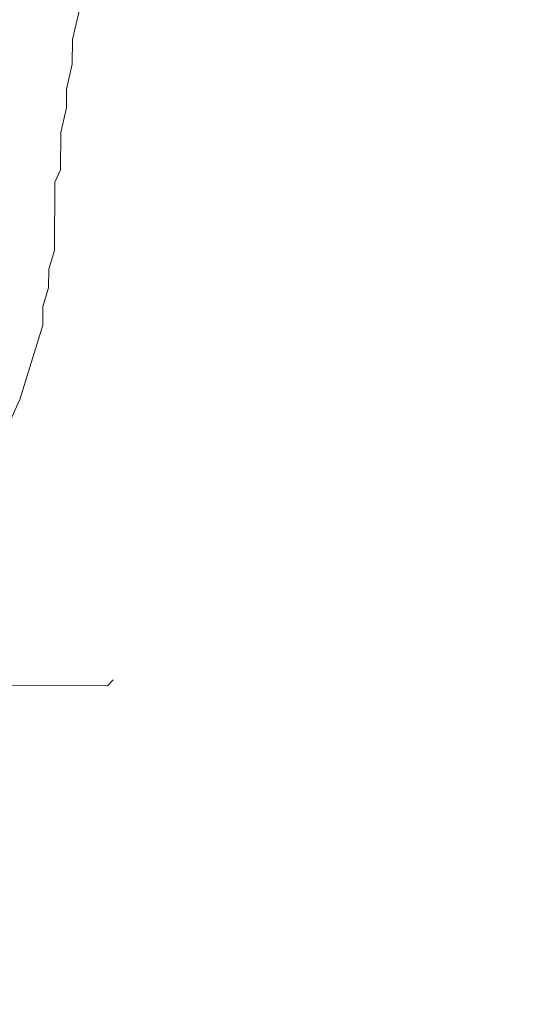
# Model space of a CAD drawing. Units: inches. Extents: x -466983 to 1020, y 324 to 318697.
# Tile 80 of 97: x 660.579 to 662.966, y 939.297 to 944.006. Entities that reach past the tile are written whole.
import ezdxf

# ---------------------------------------------------------------- set-up
doc = ezdxf.new("R2010")
doc.units = ezdxf.units.IN
doc.header["$MEASUREMENT"] = 0
doc.layers.add('A-FLOR-PATT', color=252, linetype='Continuous', lineweight=13)
doc.layers.add('A-FURN', color=8, linetype='Continuous', lineweight=18)

# ---------------------------------------------------------------- blocks, each defined once
blk = doc.blocks.new('L Shaped Sofa')
at = {"ltscale": 2}
for p, q in [((2387.3023, 747.1038), (2387.3515, 747.1578)), ((2387.3515, 747.1578), (2388.5226, 747.1523)), ((2388.1169, 744.6602), (2388.2158, 744.8766)), ((2387.9178, 744.0105), (2388.1169, 744.6602)), ((2387.9168, 743.8479), (2387.9178, 744.0105)), ((2387.867, 743.6855), (2387.9168, 743.8479)), ((2387.866, 743.5228), (2387.867, 743.6855)), ((2387.8162, 743.3604), (2387.866, 743.5228)), ((2387.8125, 742.764), (2387.8162, 743.3604)), ((2387.7631, 742.6558), (2387.8125, 742.764)), ((2387.7611, 742.3305), (2387.7631, 742.6558)), ((2387.711, 742.1139), (2387.7611, 742.3305)), ((2387.71, 741.9512), (2387.711, 742.1139)), ((2387.6598, 741.7346), (2387.71, 741.9512)), ((2387.6585, 741.5177), (2387.6598, 741.7346)), ((2387.5583, 741.0845), (2387.6585, 741.5177))]:
    blk.add_line(p, q, dxfattribs=at)

msp = doc.modelspace()

# ---------------------------------------------------------------- hatches: boundary and pattern name
at = {"layer": 'A-FLOR-PATT', "transparency": 33554572}
h = msp.add_hatch(dxfattribs=at)
h.set_pattern_fill('ANSI37', color=256, scale=30)
h.set_pattern_definition([(45, (-1212.4137, -290.035), (-2.6516504, 2.6516504), []), (135, (-1212.4137, -290.035), (-2.6516504, -2.6516504), [])])
h.paths.add_polyline_path([(901.8057, 1075.9377), (900.6144, 1075.9377), (900.6144, 1065.3856), (899.391, 1065.3856), (898.0911, 1065.3856), (892.8356, 1058.7098, -0.258377), (892.1875, 1058.3509), (879.9848, 1058.3509, -0.20177), (879.4382, 1058.5808), (874.0812, 1065.3856), (872.7813, 1065.3856), (871.5579, 1065.3856), (871.5579, 1075.9377), (813.8057, 1075.9377), (813.8057, 1044.7922), (832.3947, 1044.7922, -0.394795), (848.6602, 1028.5356), (848.6602, 1009.9377), (901.8057, 1009.9377), (901.8057, 1015.9377), (901.3057, 1015.9377), (871.3057, 1015.9377), (871.3057, 1017.2502), (871.3344, 1017.2502, -0.401453), (901.3057, 1045.9377), (901.8057, 1045.9377)])
edge = h.paths.add_edge_path(flags=16)
edge.add_line((847.7731, 1068.9486), (847.7731, 1073.7088))
edge.add_arc((849.2269, 1073.7088), 1.4538, 90, 180, ccw=False)
edge.add_line((849.2269, 1075.1627), (864.4921, 1075.1627))
edge.add_arc((864.4921, 1073.7088), 1.4538, 0, 90, ccw=False)
edge.add_line((865.9459, 1073.7088), (865.9459, 1069.0035))
edge.add_arc((832.6447, 1068.9761), 33.3012, -20.61234, 0.04725, ccw=False)
edge.add_ellipse((856.8595, 1058.48), major_axis=(0, 10.2131), ratio=0.6859192, start_angle=100.00884, end_angle=259.99116, ccw=False)
edge.add_arc((881.0742, 1068.9761), 33.3012, 180.04725, 200.61234, ccw=False)
h.paths.add_polyline_path([(853.1456, 1066.4815), (853.1456, 1066.4534), (853.1463, 1066.4534, 0.433107), (852.9166, 1066.6849), (852.9166, 1066.4534), (853.1456, 1066.4534), (853.1456, 1066.4815), (853.088, 1066.6122, 0.697939), (852.6995, 1066.4534), (852.7003, 1066.4534), (852.7003, 1066.4815), (852.9166, 1067.0012), (852.9166, 1066.6849, -0.396254)], flags=0)
h.paths.add_polyline_path([(861.0187, 1066.4815), (861.0187, 1066.4534), (861.0194, 1066.4534, 0.416404), (860.8024, 1066.6849), (860.8024, 1066.4534), (861.0187, 1066.4534), (861.0187, 1066.4815), (860.9672, 1066.6053, 0.713344), (860.5726, 1066.4534), (860.5734, 1066.4534), (860.5734, 1066.4815), (860.8024, 1067.0012), (860.8024, 1066.6849, -0.379973)], flags=0)
edge = h.paths.add_edge_path(flags=0)
edge.add_spline(control_points=[(861.1298, 1065.7855), (861.4661, 1065.2478), (861.6134, 1065.0161), (861.9833, 1064.3736), (862.1924, 1063.9443), (862.5614, 1063.0391), (862.7212, 1062.5633), (862.9865, 1061.5781), (863.092, 1061.0689), (863.2452, 1060.031), (863.293, 1059.5025), (863.3295, 1058.4409), (863.3181, 1057.9078), (863.2366, 1056.8518), (863.1664, 1056.3289), (862.9695, 1055.308), (862.8427, 1054.8099), (862.5365, 1053.8522), (862.3571, 1053.3927), (861.9514, 1052.5249), (861.7251, 1052.1166), (861.233, 1051.3622), (860.9672, 1051.0162), (860.4048, 1050.3949), (860.1082, 1050.1197), (859.4937, 1049.6461), (859.1758, 1049.4476), (858.5276, 1049.1299), (858.1973, 1049.0107), (857.5315, 1048.8518), (857.1959, 1048.8121), (856.5249, 1048.812), (856.1894, 1048.8515), (855.5236, 1049.0101), (855.1933, 1049.1291), (854.545, 1049.4465), (854.2271, 1049.6449), (853.6124, 1050.1183), (853.3158, 1050.3933), (852.7533, 1051.0143), (852.4874, 1051.3602), (851.9952, 1052.1144), (851.7688, 1052.5225), (851.3629, 1053.3902), (851.1834, 1053.8496), (850.877, 1054.8071), (850.7501, 1055.3051), (850.553, 1056.326), (850.4827, 1056.8488), (850.401, 1057.9048), (850.3895, 1058.4379), (850.4257, 1059.4995), (850.4734, 1060.0281), (850.6265, 1061.066), (850.7318, 1061.5753), (850.9969, 1062.5605), (851.1567, 1063.0365), (851.5254, 1063.9418), (851.7345, 1064.3712), (852.1056, 1065.0164), (852.2544, 1065.2503), (852.6082, 1065.7335)], knot_values=[3.915332, 3.915332, 3.915332, 3.915332, 4.013468, 4.013468, 4.175532, 4.175532, 4.337596, 4.337596, 4.49966, 4.49966, 4.661724, 4.661724, 4.823788, 4.823788, 4.985852, 4.985852, 5.147916, 5.147916, 5.30998, 5.30998, 5.472044, 5.472044, 5.634109, 5.634109, 5.796173, 5.796173, 5.958237, 5.958237, 6.120301, 6.120301, 6.282365, 6.282365, 6.444429, 6.444429, 6.606493, 6.606493, 6.768557, 6.768557, 6.930621, 6.930621, 7.092685, 7.092685, 7.254749, 7.254749, 7.416813, 7.416813, 7.578878, 7.578878, 7.740942, 7.740942, 7.903006, 7.903006, 8.06507, 8.06507, 8.227134, 8.227134, 8.389198, 8.389198, 8.551262, 8.551262, 8.65037, 8.65037, 8.65037, 8.65037], degree=3, periodic=0)
edge.add_line((852.6421, 1065.7855), (861.1298, 1065.7855))
edge = h.paths.add_edge_path(flags=0)
edge.add_ellipse((856.8496, 1057.7432), major_axis=(0, 7.7921), ratio=0.687861, start_angle=0, end_angle=360)
h.paths.add_polyline_path([(848.8634, 1069.3891), (848.8634, 1073.9605, -0.414214), (849.9538, 1075.0508), (863.7652, 1075.0508, -0.414214), (864.8555, 1073.9605), (864.8555, 1069.3891, -0.388936), (864.5237, 1069.027, -0.043561), (849.1953, 1069.027, -0.388936)], flags=0)
h.paths.add_polyline_path([(853.1006, 1068.1122, -1), (852.6775, 1068.1122, -1)], flags=0)
edge = h.paths.add_edge_path(flags=0)
edge.add_ellipse((856.8595, 1057.3378), major_axis=(0, 2.207), ratio=0.657164, start_angle=0, end_angle=360)
h.paths.add_polyline_path([(861.0415, 1068.1122, -1), (860.6184, 1068.1122, -1)], flags=0)
edge = h.paths.add_edge_path()
edge.add_line((573.9537, 1057.3412), (573.9537, 1075.9377))
edge.add_line((573.9537, 1075.9377), (558.7308, 1075.9377))
edge.add_line((558.7308, 1075.9377), (558.7308, 1065.3856))
edge.add_line((558.7308, 1065.3856), (557.5074, 1065.3856))
edge.add_line((557.5074, 1065.3856), (556.2075, 1065.3856))
edge.add_line((556.2075, 1065.3856), (550.952, 1058.7098))
edge.add_arc((550.3039, 1059.1155), 0.7646, 270, 327.9483, ccw=False)
edge.add_line((550.3039, 1058.3509), (538.1012, 1058.3509))
edge.add_arc((538.1012, 1059.1155), 0.7646, 224.3704, 270, ccw=False)
edge.add_line((537.5546, 1058.5808), (532.1976, 1065.3856))
edge.add_line((532.1976, 1065.3856), (530.8977, 1065.3856))
edge.add_line((530.8977, 1065.3856), (529.6743, 1065.3856))
edge.add_line((529.6743, 1065.3856), (529.6743, 1075.9377))
edge.add_line((529.6743, 1075.9377), (520.8057, 1075.9377))
edge.add_line((520.8057, 1075.9377), (520.8057, 1045.9377))
edge.add_line((520.8057, 1045.9377), (521.3057, 1045.9377))
edge.add_arc((521.3057, 1015.9377), 30, 2.50749, 90, ccw=False)
edge.add_line((551.277, 1017.2502), (551.3057, 1017.2502))
edge.add_line((551.3057, 1017.2502), (551.3057, 1015.9377))
edge.add_line((551.3057, 1015.9377), (520.8057, 1015.9377))
edge.add_line((520.8057, 1015.9377), (520.8057, 1009.9377))
edge.add_line((520.8057, 1009.9377), (559.1913, 1010.4022))
edge.add_arc((559.1913, 1011.856), 1.4538, 180, 270, ccw=False)
edge.add_line((557.7375, 1011.856), (557.7375, 1016.5613))
edge.add_arc((591.0386, 1016.5888), 33.3012, 159.38766, 180.04725, ccw=False)
edge.add_ellipse((566.8239, 1027.0848), major_axis=(0, 10.2131), ratio=0.6859192, start_angle=280.00884, end_angle=439.99116, ccw=False)
edge.add_arc((542.6091, 1016.5888), 33.3012, 0.04725, 20.61234, ccw=False)
edge.add_line((575.9103, 1016.6162), (575.9103, 1011.856))
edge.add_arc((574.4565, 1011.856), 1.4538, -90, 0, ccw=False)
edge.add_line((574.4565, 1010.4022), (608.8057, 1009.9377))
edge.add_line((608.8057, 1009.9377), (608.8057, 1041.0857))
edge.add_line((608.8057, 1041.0857), (590.2179, 1041.0857))
edge.add_arc((590.775, 1057.9074), 16.8309, 181.92775, 268.10321, ccw=False)
edge = h.paths.add_edge_path()
edge.add_ellipse((494.2443, 583.6204), major_axis=(0, 10.2131), ratio=0.6859192, start_angle=280.00884, end_angle=439.99116, ccw=False)
edge.add_arc((470.0296, 573.1243), 33.3012, 0.04725, 20.61234, ccw=False)
edge.add_line((503.3307, 573.1518), (503.3307, 568.3916))
edge.add_arc((501.8769, 568.3916), 1.4538, -90, 0, ccw=False)
edge.add_line((501.8769, 566.9377), (539.8057, 566.9377))
edge.add_line((539.8057, 566.9377), (539.8057, 572.9377))
edge.add_line((539.8057, 572.9377), (539.3057, 572.9377))
edge.add_line((539.3057, 572.9377), (509.3057, 572.9377))
edge.add_line((509.3057, 572.9377), (509.3057, 574.2502))
edge.add_line((509.3057, 574.2502), (509.3344, 574.2502))
edge.add_arc((539.3057, 572.9377), 30, 90, 177.49251, ccw=False)
edge.add_line((539.3057, 602.9377), (539.8057, 602.9377))
edge.add_line((539.8057, 602.9377), (539.8057, 626.9377))
edge.add_line((539.8057, 626.9377), (531.7718, 626.9377))
edge.add_line((531.7718, 626.9377), (531.7718, 616.3856))
edge.add_line((531.7718, 616.3856), (530.5484, 616.3856))
edge.add_line((530.5484, 616.3856), (529.2485, 616.3856))
edge.add_line((529.2485, 616.3856), (523.7105, 609.3509))
edge.add_line((523.7105, 609.3509), (510.7766, 609.3509))
edge.add_line((510.7766, 609.3509), (505.2386, 616.3856))
edge.add_line((505.2386, 616.3856), (503.9387, 616.3856))
edge.add_line((503.9387, 616.3856), (502.7153, 616.3856))
edge.add_line((502.7153, 616.3856), (502.7153, 626.9377))
edge.add_line((502.7153, 626.9377), (481.6983, 626.9377))
edge.add_line((481.6983, 626.9377), (481.6983, 610.995))
edge.add_arc((467.2703, 611.4728), 14.4359, 271.92775, 358.10321, ccw=False)
edge.add_line((467.7559, 597.0451), (451.8057, 597.0451))
edge.add_line((451.8057, 597.0451), (451.8057, 584.4035))
edge.add_line((451.8057, 584.4035), (451.8057, 566.9377))
edge.add_line((451.8057, 566.9377), (486.6117, 566.9377))
edge.add_arc((486.6117, 568.3916), 1.4538, 180, 270, ccw=False)
edge.add_line((485.1579, 568.3916), (485.1579, 573.0969))
edge.add_arc((518.4591, 573.1243), 33.3012, 159.38766, 180.04725, ccw=False)
h.paths.add_polyline_path([(836.2609, 1020.7328), (879.8898, 1020.7328), (879.8898, 1039.3902), (836.2609, 1039.3902)], flags=25)
h.paths.add_polyline_path([(549.9851, 1036.7492), (593.614, 1036.7492), (593.614, 1055.4065), (549.9851, 1055.4065)], flags=24)
h.paths.add_polyline_path([(475.123, 595.5959), (518.752, 595.5959), (518.752, 614.2532), (475.123, 614.2532)], flags=24)
h = msp.add_hatch(dxfattribs=at)
h.set_pattern_fill('ANSI37', color=256, scale=20)
h.set_pattern_definition([(45, (-1212.4137, -290.035), (-1.767767, 1.767767), []), (135, (-1212.4137, -290.035), (-1.767767, -1.767767), [])])
h.paths.add_polyline_path([(809.8057, 870.9377), (809.8057, 888.1519), (806.9985, 888.1519), (802.6624, 888.1519), (789.3832, 888.1519), (786.2846, 888.1519, -0.414214), (785.4991, 888.9374), (785.4991, 900.1959), (785.4991, 908.4696, -0.414214), (786.8082, 909.7787, -0.414214), (785.4991, 911.0878), (785.4991, 929.1015, -0.414214), (786.8082, 930.4106, -0.414214), (785.4991, 931.7197), (785.4991, 931.9039, -0.414214), (784.19, 930.5948), (766.7223, 930.5948, -0.412359), (765.4132, 931.8956, -0.413741), (764.1145, 930.5782), (744.5781, 930.422, -0.416556), (743.7864, 931.2075), (743.7864, 933.5153), (742.2154, 933.5153), (742.2154, 952.024, -0.001344), (743.7864, 952.1998), (743.7864, 953.9377), (678.5915, 953.9377), (678.5915, 951.1305), (678.5915, 946.7945), (678.5915, 933.5153), (678.5915, 930.4166, -0.414214), (677.806, 929.6312), (666.5475, 929.6312), (658.2738, 929.6312, -0.414214), (656.9647, 930.9403, -0.414214), (655.6556, 929.6312), (637.6419, 929.6312, -0.414214), (636.3328, 930.9403, -0.414214), (635.0237, 929.6312), (634.8395, 929.6312, -0.414214), (636.1486, 928.322), (636.1486, 910.8544, -0.412359), (634.8478, 909.5452, -0.413741), (636.1653, 908.2466), (636.3214, 888.7102, -0.416556), (635.5359, 887.9184), (633.2281, 887.9184), (633.2281, 886.3475), (614.7194, 886.3475, -0.001344), (614.5436, 887.9184), (612.8057, 887.9184), (612.8057, 834.9377), (612.8057, 752.9377), (612.8057, 748.9377), (612.8057, 697.9377), (654.8057, 697.9377), (654.8057, 701.9377), (715.8057, 701.9377), (715.8057, 737.4353), (774.2918, 737.4353), (774.2918, 795.9377), (809.8057, 795.9377)])
h.paths.add_polyline_path([(679.2761, 849.5757, 0.102523), (682.1475, 849.2608, -0.080461), (694.5428, 849.7725, -0.283899), (694.4822, 849.0082, 0.136605), (694.4068, 848.8103, -0.030441), (694.5428, 846.8929), (694.5428, 842.6198), (694.5428, 838.3466, -0.028219), (694.4246, 836.5684), (694.425, 836.5684, 0.196187), (694.4456, 836.2708, -0.302897), (694.5428, 835.467, -0.080461), (682.1475, 835.9787, 0.102523), (679.2761, 835.6638, -0.58611), (678.6457, 836.0169), (678.6457, 849.2227, -0.58611)], flags=16)
h.paths.add_polyline_path([(679.5173, 848.6515, 0.699597), (679.476, 848.6342, 1.20716), (679.1935, 848.7422, 0.010621)], flags=0)
h.paths.add_polyline_path([(679.4923, 836.5608, -0.013798), (679.9178, 836.6594, -0.071703), (682.8533, 837.1434, -0.165743), (682.1665, 839.1006), (682.1665, 842.6094), (682.1665, 846.0603, -0.240616), (683.4733, 848.6767, -0.068263), (693.9295, 849.0082), (693.7875, 848.7083), (693.7875, 849.0228, 0.067332), (683.4733, 848.6767, 0.240616), (682.1665, 846.0603), (682.1665, 842.6094), (682.1665, 839.1006, 0.23459), (683.461, 836.5513, 0.068093), (693.7875, 836.1955), (693.7875, 836.5104), (693.9296, 836.2102, -0.077215), (682.2421, 836.7815, 0.086627), (679.5283, 836.5701, -0.628402), (679.5029, 836.5735), (679.5029, 836.6071, 0.910458)], flags=0)
h.paths.add_polyline_path([(679.476, 848.6364), (679.2069, 848.647), (679.2069, 836.5718, 0.913566), (679.3645, 836.5861), (679.476, 836.5824)], flags=0)
h.paths.add_polyline_path([(679.2761, 829.8604, 0.102523), (682.1475, 829.5455, -0.080461), (694.5428, 830.0572, -0.283899), (694.4822, 829.2929, 0.136605), (694.4068, 829.095, -0.030441), (694.5428, 827.1776), (694.5428, 822.9045), (694.5428, 818.6314, -0.028219), (694.4246, 816.8531), (694.425, 816.8532, 0.196187), (694.4456, 816.5555, -0.302897), (694.5428, 815.7517, -0.080461), (682.1475, 816.2635, 0.102523), (679.2761, 815.9485, -0.58611), (678.6457, 816.3016), (678.6457, 829.5074, -0.58611)], flags=16)
h.paths.add_polyline_path([(679.5173, 828.9362, 0.699597), (679.476, 828.9189, 1.20716), (679.1935, 829.0269, 0.010621)], flags=0)
h.paths.add_polyline_path([(679.4923, 816.8456, -0.013798), (679.9178, 816.9441, -0.071703), (682.8533, 817.4281, -0.165743), (682.1665, 819.3853), (682.1665, 822.8941), (682.1665, 826.345, -0.240616), (683.4733, 828.9614, -0.068263), (693.9295, 829.2929), (693.7875, 828.9931), (693.7875, 829.3076, 0.067332), (683.4733, 828.9614, 0.240616), (682.1665, 826.345), (682.1665, 822.8941), (682.1665, 819.3853, 0.23459), (683.461, 816.836, 0.068093), (693.7875, 816.4802), (693.7875, 816.7952), (693.9296, 816.4949, -0.077215), (682.2421, 817.0662, 0.086627), (679.5283, 816.8549, -0.628402), (679.5029, 816.8582), (679.5029, 816.8918, 0.910458)], flags=0)
h.paths.add_polyline_path([(679.476, 828.9211), (679.2069, 828.9317), (679.2069, 816.8565, 0.913566), (679.3645, 816.8708), (679.476, 816.8671)], flags=0)
h.paths.add_polyline_path([(679.2761, 810.1451, 0.102523), (682.1475, 809.8302, -0.080461), (694.5428, 810.342, -0.3023), (694.4466, 809.5394, 0.10023), (694.4058, 809.3878, -0.03057), (694.5428, 807.4623), (694.5428, 803.1892), (694.5428, 798.9161, -0.03057), (694.4058, 796.9906, 0.10023), (694.4466, 796.839, -0.3023), (694.5428, 796.0365, -0.080461), (682.1475, 796.5482, 0.102523), (679.2761, 796.2333, -0.58611), (678.6457, 796.5863), (678.6457, 809.7921, -0.58611)], flags=16)
h.paths.add_polyline_path([(679.5173, 809.2417, 0.699597), (679.476, 809.2244, 1.20716), (679.1935, 809.3324, 0.010621)], flags=0)
h.paths.add_polyline_path([(679.4923, 797.151, -0.013798), (679.9178, 797.2496, -0.071703), (682.8533, 797.7336, -0.165743), (682.1665, 799.6908), (682.1665, 803.1996), (682.1665, 806.6505, -0.239349), (683.461, 809.2577, -0.072465), (694.4468, 809.5405, 0.197932), (694.425, 809.2405), (693.7875, 809.2985), (693.7875, 809.6135, 0.068093), (683.461, 809.2577, 0.239349), (682.1665, 806.6505), (682.1665, 803.1996), (682.1665, 799.6908, 0.235854), (683.4733, 797.1323, 0.067332), (693.7875, 796.7861), (693.7875, 797.1006), (694.425, 797.1586, 0.197932), (694.4468, 796.8586, -0.080419), (682.1557, 797.3795, 0.083867), (679.5283, 797.1603, -0.628402), (679.5029, 797.1637), (679.5029, 797.1973, 0.910458)], flags=0)
h.paths.add_polyline_path([(679.2069, 809.2372), (679.2069, 797.162, 0.913566), (679.3645, 797.1763), (679.476, 797.1726), (679.476, 809.2266)], flags=0)
h.paths.add_polyline_path([(695.3643, 853.2989), (728.2231, 853.2989), (728.2231, 771.1519), (695.3643, 771.1519)], flags=16)
h.paths.add_polyline_path([(696.0215, 852.6417), (727.5659, 852.6417), (727.5659, 771.809), (696.0215, 771.809)], flags=0)
h.paths.add_polyline_path([(679.2761, 788.7869, 0.102523), (682.1475, 788.472, -0.080461), (694.5428, 788.9837, -0.3023), (694.4466, 788.1812, 0.10023), (694.4058, 788.0296, -0.03057), (694.5428, 786.1041), (694.5428, 781.831), (694.5428, 777.5578, -0.03057), (694.4058, 775.6323, 0.10023), (694.4466, 775.4808, -0.3023), (694.5428, 774.6782, -0.080461), (682.1475, 775.19, 0.102523), (679.2761, 774.875, -0.58611), (678.6457, 775.2281), (678.6457, 788.4339, -0.58611)], flags=16)
h.paths.add_polyline_path([(679.5173, 787.8834, 0.699597), (679.476, 787.8662, 1.20716), (679.1935, 787.9742, 0.010621)], flags=0)
h.paths.add_polyline_path([(679.4923, 775.7928, -0.013798), (679.9178, 775.8914, -0.071703), (682.8533, 776.3753, -0.165743), (682.1665, 778.3325), (682.1665, 781.8414), (682.1665, 785.2922, -0.239349), (683.461, 787.8995, -0.072465), (694.4468, 788.1823, 0.197932), (694.425, 787.8823), (693.7875, 787.9403), (693.7875, 788.2553, 0.068093), (683.461, 787.8995, 0.239349), (682.1665, 785.2922), (682.1665, 781.8414), (682.1665, 778.3325, 0.235854), (683.4733, 775.7741, 0.067332), (693.7875, 775.4279), (693.7875, 775.7424), (694.425, 775.8004, 0.197932), (694.4468, 775.5004, -0.080419), (682.1557, 776.0212, 0.083867), (679.5283, 775.8021, -0.628402), (679.5029, 775.8054), (679.5029, 775.8391, 0.910458)], flags=0)
h.paths.add_polyline_path([(679.2069, 787.8789), (679.2069, 775.8038, 0.913566), (679.3645, 775.818), (679.476, 775.8144), (679.476, 787.8684)], flags=0)
h.paths.add_polyline_path([(704.641, 854.1204, -0.080461), (705.1527, 866.5157, 0.102523), (704.8378, 869.3871, -0.58611), (705.1908, 870.0174), (718.3966, 870.0174, -0.58611), (718.7496, 869.3871, 0.102523), (718.4347, 866.5157, -0.080461), (718.9465, 854.1204, -0.3023), (718.1439, 854.2166, 0.10023), (717.9924, 854.2574, -0.03057), (716.0668, 854.1204), (711.7937, 854.1204), (707.5206, 854.1204, -0.03057), (705.5951, 854.2574, 0.10023), (705.4435, 854.2166, -0.3023)], flags=16)
h.paths.add_polyline_path([(717.8462, 869.1459, 0.699597), (717.8289, 869.1872, 1.20716), (717.9369, 869.4697, 0.010621)], flags=0)
h.paths.add_polyline_path([(705.4631, 854.2164, -0.080419), (705.984, 866.5074, 0.083867), (705.7648, 869.1349, -0.628402), (705.7682, 869.1603), (705.8018, 869.1603, 0.910458), (705.7555, 869.1709, -0.013798), (705.8541, 868.7454, -0.071703), (706.3381, 865.8099, -0.165743), (708.2953, 866.4967), (711.8041, 866.4967), (715.255, 866.4967, -0.239349), (717.8622, 865.2022, -0.072465), (718.145, 854.2164, 0.197932), (717.845, 854.2382), (717.903, 854.8757), (718.218, 854.8757, 0.068093), (717.8622, 865.2022, 0.239349), (715.255, 866.4967), (711.8041, 866.4967), (708.2953, 866.4967, 0.235854), (705.7368, 865.1898, 0.067332), (705.3906, 854.8757), (705.7051, 854.8757), (705.7631, 854.2382, 0.197932)], flags=16)
h.paths.add_polyline_path([(705.7665, 869.4563, 0.913566), (705.7808, 869.2987), (705.7771, 869.1872), (717.8311, 869.1872), (717.8417, 869.4563)], flags=0)
h.paths.add_polyline_path([(729.0446, 842.6198), (729.0446, 846.8929, -0.03057), (729.1817, 848.8184, 0.10023), (729.1408, 848.9699, -0.3023), (729.0446, 849.7725, -0.080461), (741.4399, 849.2608, 0.102523), (744.3113, 849.5757, -0.58611), (744.9417, 849.2227), (744.9417, 836.0169, -0.58611), (744.3113, 835.6638, 0.102523), (741.4399, 835.9787, -0.080461), (729.0446, 835.467, -0.3023), (729.1408, 836.2696, 0.10023), (729.1817, 836.4211, -0.03057), (729.0446, 838.3466)], flags=16)
h.paths.add_polyline_path([(744.1115, 836.5846, 1.20716), (744.3939, 836.4766, 0.010621), (744.0701, 836.5673, 0.699597)], flags=0)
h.paths.add_polyline_path([(729.1407, 836.2684, 0.197932), (729.1624, 836.5684), (729.7999, 836.5104), (729.7999, 836.1955, 0.068093), (740.1264, 836.5513, 0.239349), (741.4209, 839.1585), (741.4209, 842.6094), (741.4209, 846.1182, 0.235854), (740.1141, 848.6767, 0.067332), (729.7999, 849.0228), (729.7999, 848.7083), (729.1624, 848.6503, 0.197932), (729.1407, 848.9504, -0.080419), (741.4317, 848.4295, 0.083867), (744.0591, 848.6486, -0.628402), (744.0845, 848.6453), (744.0845, 848.6117, 0.910458), (744.0951, 848.6579, -0.013798), (743.6696, 848.5594, -0.071703), (740.7341, 848.0754, -0.165743), (741.4209, 846.1182), (741.4209, 842.6094), (741.4209, 839.1585, -0.239349), (740.1264, 836.5513, -0.072465)], flags=0)
h.paths.add_polyline_path([(729.0446, 830.0572, -0.080461), (741.4399, 829.5455, 0.102523), (744.3113, 829.8604, -0.58611), (744.9417, 829.5074), (744.9417, 816.3016, -0.58611), (744.3113, 815.9485, 0.102523), (741.4399, 816.2635, -0.080461), (729.0446, 815.7517, -0.3023), (729.1408, 816.5543, 0.10023), (729.1817, 816.7058, -0.03057), (729.0446, 818.6314), (729.0446, 822.9045), (729.0446, 827.1776, -0.03057), (729.1817, 829.1031, 0.10023), (729.1408, 829.2547, -0.3023)], flags=16)
h.paths.add_polyline_path([(744.1115, 816.8693, 1.20716), (744.3939, 816.7613, 0.010621), (744.0701, 816.852, 0.699597)], flags=0)
h.paths.add_polyline_path([(729.1407, 829.2351, -0.080419), (741.4317, 828.7142, 0.083867), (744.0591, 828.9334, -0.628402), (744.0845, 828.93), (744.0845, 828.8964, 0.910458), (744.0951, 828.9427, -0.013798), (743.6696, 828.8441, -0.071703), (740.7341, 828.3601, -0.165743), (741.4209, 826.4029), (741.4209, 822.8941), (741.4209, 819.4432, -0.239349), (740.1264, 816.836, -0.072465), (729.1407, 816.5531, 0.197932), (729.1624, 816.8532), (729.7999, 816.7952), (729.7999, 816.4802, 0.068093), (740.1264, 816.836, 0.239349), (741.4209, 819.4432), (741.4209, 822.8941), (741.4209, 826.4029, 0.235854), (740.1141, 828.9614, 0.067332), (729.7999, 829.3076), (729.7999, 828.9931), (729.1624, 828.9351, 0.197932)], flags=16)
h.paths.add_polyline_path([(729.0446, 810.342, -0.080461), (741.4399, 809.8302, 0.102523), (744.3113, 810.1451, -0.58611), (744.9417, 809.7921), (744.9417, 796.5863, -0.58611), (744.3113, 796.2333, 0.102523), (741.4399, 796.5482, -0.080461), (729.0446, 796.0365, -0.283899), (729.1052, 796.8007, 0.136605), (729.1806, 796.9987, -0.030441), (729.0446, 798.9161), (729.0446, 803.1892), (729.0446, 807.4623, -0.028219), (729.1628, 809.2406), (729.1624, 809.2405, 0.196187), (729.1418, 809.5382, -0.302897)], flags=16)
h.paths.add_polyline_path([(744.1115, 797.1748, 1.20716), (744.3939, 797.0668, 0.010621), (744.0701, 797.1575, 0.699597)], flags=0)
h.paths.add_polyline_path([(741.3453, 809.0275, 0.086627), (744.0591, 809.2388, -0.628402), (744.0845, 809.2355), (744.0845, 809.2019, 0.910458), (744.0951, 809.2481, -0.013798), (743.6696, 809.1496, -0.071703), (740.7341, 808.6656, -0.165743), (741.4209, 806.7084), (741.4209, 803.1996), (741.4209, 799.7487, -0.240616), (740.1141, 797.1323, -0.068263), (729.658, 796.8008), (729.7999, 797.1006), (729.7999, 796.7861, 0.067332), (740.1141, 797.1323, 0.240616), (741.4209, 799.7487), (741.4209, 803.1996), (741.4209, 806.7084, 0.23459), (740.1264, 809.2577, 0.068093), (729.7999, 809.6135), (729.7999, 809.2985), (729.6578, 809.5988, -0.077215)], flags=0)
h.paths.add_polyline_path([(704.641, 770.3304, -0.283899), (705.4053, 770.2697, 0.136605), (705.6032, 770.1944, -0.030441), (707.5206, 770.3304), (711.7937, 770.3304), (716.0668, 770.3304, -0.028219), (717.8451, 770.2122), (717.845, 770.2126, 0.196187), (718.1427, 770.2331, -0.302897), (718.9465, 770.3304, -0.080461), (718.4347, 757.9351, 0.102523), (718.7496, 755.0637, -0.58611), (718.3966, 754.4333), (705.1908, 754.4333, -0.58611), (704.8378, 755.0637, 0.102523), (705.1527, 757.9351, -0.080461)], flags=16)
h.paths.add_polyline_path([(705.762, 755.3048, 0.699597), (705.7793, 755.2635, 1.20716), (705.6713, 754.9811, 0.010621)], flags=0)
h.paths.add_polyline_path([(705.4053, 769.717), (705.7051, 769.5751), (705.3906, 769.5751, 0.067332), (705.7368, 759.2609, 0.240616), (708.3532, 757.954), (711.8041, 757.954), (715.3129, 757.954, 0.23459), (717.8622, 759.2485, 0.068093), (718.218, 769.5751), (717.903, 769.5751), (718.2033, 769.7172, -0.077215), (717.632, 758.0297, 0.086627), (717.8433, 755.3159, -0.628402), (717.84, 755.2904), (717.8064, 755.2904, 0.910458), (717.8526, 755.2799, -0.013798), (717.7541, 755.7053, -0.071703), (717.2701, 758.6409, -0.165743), (715.3129, 757.954), (711.8041, 757.954), (708.3532, 757.954, -0.240616), (705.7368, 759.2609, -0.068263)], flags=0)
h.paths.add_polyline_path([(729.0446, 788.9837, -0.080461), (741.4399, 788.472, 0.102523), (744.3113, 788.7869, -0.58611), (744.9417, 788.4339), (744.9417, 775.2281, -0.58611), (744.3113, 774.875, 0.102523), (741.4399, 775.19, -0.080461), (729.0446, 774.6782, -0.283899), (729.1052, 775.4425, 0.136605), (729.1806, 775.6405, -0.030441), (729.0446, 777.5578), (729.0446, 781.831), (729.0446, 786.1041, -0.028219), (729.1628, 787.8823), (729.1624, 787.8823, 0.196187), (729.1418, 788.1799, -0.302897)], flags=16)
h.paths.add_polyline_path([(744.1115, 775.8165, 1.20716), (744.3939, 775.7086, 0.010621), (744.0701, 775.7993, 0.699597)], flags=0)
h.paths.add_polyline_path([(741.3453, 787.6692, 0.086627), (744.0591, 787.8806, -0.628402), (744.0845, 787.8773), (744.0845, 787.8437, 0.910458), (744.0951, 787.8899, -0.013798), (743.6696, 787.7913, -0.071703), (740.7341, 787.3074, -0.165743), (741.4209, 785.3502), (741.4209, 781.8414), (741.4209, 778.3905, -0.240616), (740.1141, 775.7741, -0.068263), (729.658, 775.4425), (729.7999, 775.7424), (729.7999, 775.4279, 0.067332), (740.1141, 775.7741, 0.240616), (741.4209, 778.3905), (741.4209, 781.8414), (741.4209, 785.3502, 0.23459), (740.1264, 787.8995, 0.068093), (729.7999, 788.2553), (729.7999, 787.9403), (729.6578, 788.2405, -0.077215)], flags=0)
h.paths.add_polyline_path([(744.1115, 848.6364), (744.1115, 836.5824), (744.3805, 836.5718), (744.3805, 848.647, 0.913566), (744.2229, 848.6327)], flags=0)
h.paths.add_polyline_path([(744.2229, 828.9174), (744.1115, 828.9211), (744.1115, 816.8671), (744.3805, 816.8565), (744.3805, 828.9317, 0.913566)], flags=0)
h.paths.add_polyline_path([(717.8311, 755.2635), (705.7771, 755.2635), (705.7665, 754.9945), (717.8417, 754.9945, 0.913566), (717.8274, 755.1521)], flags=0)
h.paths.add_polyline_path([(744.2229, 809.2229), (744.1115, 809.2266), (744.1115, 797.1726), (744.3805, 797.162), (744.3805, 809.2372, 0.913566)], flags=0)
h.paths.add_polyline_path([(744.1115, 787.8684), (744.1115, 775.8144), (744.3805, 775.8038), (744.3805, 787.8789, 0.913566), (744.2229, 787.8647)], flags=0)
h.paths.add_polyline_path([(678.8774, 877.1228), (737.6127, 877.1228), (737.6127, 899.5116), (678.8774, 899.5116)], flags=24)

# ---------------------------------------------------------------- linework, layer by layer
at = {"layer": 'A-FURN', "ltscale": 2}
for p, q in [((660.8867, 944.1493), (660.8317, 943.9118)), ((660.8867, 944.1493), (660.8317, 943.9118)), ((660.8867, 944.1493), (660.8317, 943.9118)), ((660.8867, 944.1493), (660.8317, 943.9118)), ((660.8867, 944.1493), (660.8317, 943.9118)), ((660.8867, 944.1493), (660.8317, 943.9118)), ((660.8317, 943.9118), (660.831, 943.7929)), ((660.8317, 943.9118), (660.831, 943.7929)), ((660.8317, 943.9118), (660.831, 943.7929)), ((660.8317, 943.9118), (660.831, 943.7929)), ((660.8317, 943.9118), (660.831, 943.7929)), ((660.8317, 943.9118), (660.831, 943.7929)), ((660.831, 943.7929), (660.8035, 943.6741)), ((660.831, 943.7929), (660.8035, 943.6741)), ((660.831, 943.7929), (660.8035, 943.6741)), ((660.831, 943.7929), (660.8035, 943.6741)), ((660.831, 943.7929), (660.8035, 943.6741)), ((660.831, 943.7929), (660.8035, 943.6741)), ((660.8035, 943.6741), (660.8029, 943.585)), ((660.8035, 943.6741), (660.8029, 943.585)), ((660.8035, 943.6741), (660.8029, 943.585)), ((660.8035, 943.6741), (660.8029, 943.585)), ((660.8035, 943.6741), (660.8029, 943.585)), ((660.8035, 943.6741), (660.8029, 943.585)), ((660.8029, 943.585), (660.7755, 943.4662)), ((660.8029, 943.585), (660.7755, 943.4662)), ((660.8029, 943.585), (660.7755, 943.4662)), ((660.8029, 943.585), (660.7755, 943.4662)), ((660.8029, 943.585), (660.7755, 943.4662)), ((660.8029, 943.585), (660.7755, 943.4662)), ((660.7755, 943.4662), (660.7744, 943.2879)), ((660.7755, 943.4662), (660.7744, 943.2879)), ((660.7755, 943.4662), (660.7744, 943.2879)), ((660.7755, 943.4662), (660.7744, 943.2879)), ((660.7755, 943.4662), (660.7744, 943.2879)), ((660.7755, 943.4662), (660.7744, 943.2879)), ((660.7744, 943.2879), (660.7473, 943.2286)), ((660.7744, 943.2879), (660.7473, 943.2286)), ((660.7744, 943.2879), (660.7473, 943.2286)), ((660.7744, 943.2879), (660.7473, 943.2286)), ((660.7744, 943.2879), (660.7473, 943.2286)), ((660.7744, 943.2879), (660.7473, 943.2286)), ((660.7473, 943.2286), (660.7453, 942.9016)), ((660.7473, 943.2286), (660.7453, 942.9016)), ((660.7473, 943.2286), (660.7453, 942.9016)), ((660.7473, 943.2286), (660.7453, 942.9016)), ((660.7473, 943.2286), (660.7453, 942.9016)), ((660.7473, 943.2286), (660.7453, 942.9016)), ((660.7453, 942.9016), (660.718, 942.8126)), ((660.7453, 942.9016), (660.718, 942.8126)), ((660.7453, 942.9016), (660.718, 942.8126)), ((660.7453, 942.9016), (660.718, 942.8126)), ((660.7453, 942.9016), (660.718, 942.8126)), ((660.7453, 942.9016), (660.718, 942.8126)), ((660.718, 942.8126), (660.7174, 942.7234)), ((660.718, 942.8126), (660.7174, 942.7234)), ((660.718, 942.8126), (660.7174, 942.7234)), ((660.718, 942.8126), (660.7174, 942.7234)), ((660.718, 942.8126), (660.7174, 942.7234)), ((660.718, 942.8126), (660.7174, 942.7234)), ((660.7174, 942.7234), (660.6901, 942.6344)), ((660.7174, 942.7234), (660.6901, 942.6344)), ((660.7174, 942.7234), (660.6901, 942.6344)), ((660.7174, 942.7234), (660.6901, 942.6344)), ((660.7174, 942.7234), (660.6901, 942.6344)), ((660.7174, 942.7234), (660.6901, 942.6344)), ((660.6901, 942.6344), (660.6896, 942.5452)), ((660.6901, 942.6344), (660.6896, 942.5452)), ((660.6901, 942.6344), (660.6896, 942.5452)), ((660.6901, 942.6344), (660.6896, 942.5452)), ((660.6901, 942.6344), (660.6896, 942.5452)), ((660.6901, 942.6344), (660.6896, 942.5452)), ((660.6896, 942.5452), (660.5804, 942.189)), ((660.6896, 942.5452), (660.5804, 942.189)), ((660.6896, 942.5452), (660.5804, 942.189)), ((660.6896, 942.5452), (660.5804, 942.189)), ((660.6896, 942.5452), (660.5804, 942.189)), ((660.6896, 942.5452), (660.5804, 942.189)), ((660.5804, 942.189), (660.5262, 942.0704)), ((660.5804, 942.189), (660.5262, 942.0704)), ((660.5804, 942.189), (660.5262, 942.0704)), ((660.5804, 942.189), (660.5262, 942.0704)), ((660.5804, 942.189), (660.5262, 942.0704)), ((660.5804, 942.189), (660.5262, 942.0704)), ((661, 940.8198), (660.358, 940.8228)), ((661, 940.8198), (660.358, 940.8228)), ((661, 940.8198), (660.358, 940.8228)), ((661, 940.8198), (660.358, 940.8228)), ((661, 940.8198), (660.358, 940.8228)), ((661, 940.8198), (660.358, 940.8228)), ((661.027, 940.8494), (661, 940.8198)), ((661.027, 940.8494), (661, 940.8198)), ((661.027, 940.8494), (661, 940.8198)), ((661.027, 940.8494), (661, 940.8198)), ((661.027, 940.8494), (661, 940.8198)), ((661.027, 940.8494), (661, 940.8198))]:
    msp.add_line(p, q, dxfattribs=at)

# ---------------------------------------------------------------- block references
at = {"layer": 'A-FURN', "xscale": 0.5482153745360612, "yscale": 0.5482153745360612, "zscale": 0.5482153745360612, "rotation": 180}
msp.add_blockref('L Shaped Sofa', (1969.7828, 1350.4232), dxfattribs=at)

doc.saveas('drawing.dxf')
